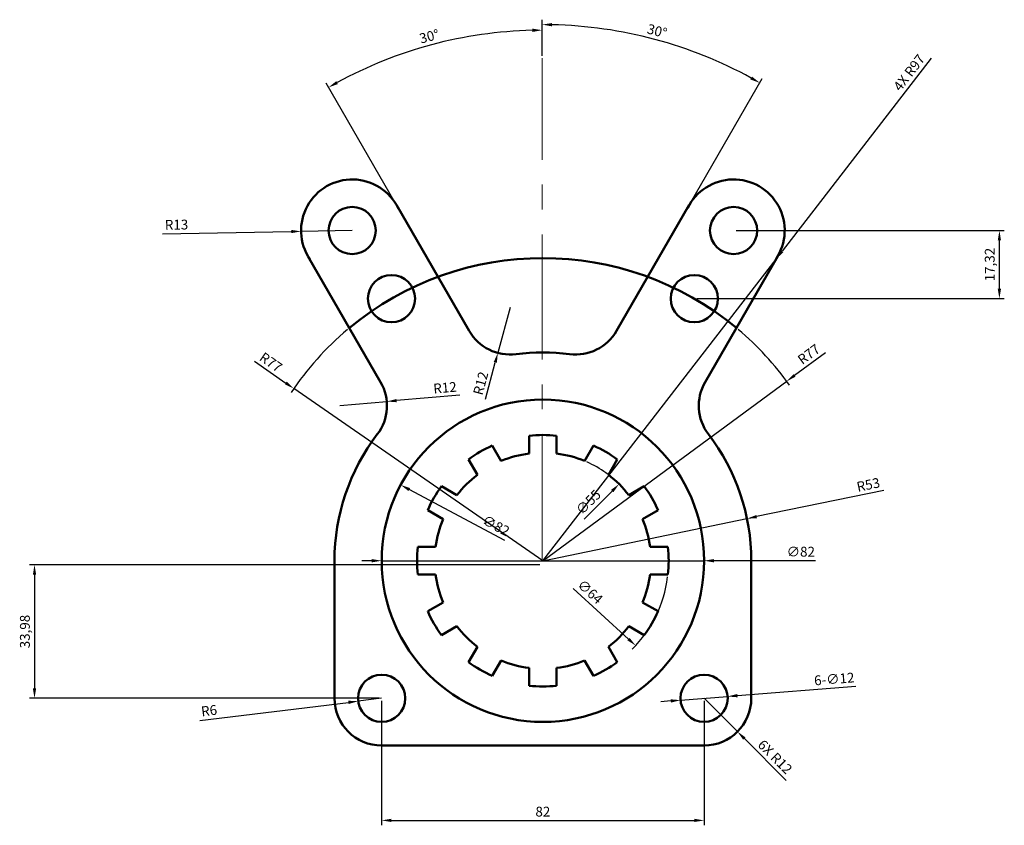
# Model space of a CAD drawing. Units: millimetres. Extents: x 2412 to 2662, y 1652 to 1857.
import ezdxf

# ---------------------------------------------------------------- set-up
doc = ezdxf.new("R2010")
doc.units = ezdxf.units.MM
doc.linetypes.add('CENTER', pattern=[50.8, 31.75, -6.35, 6.35, -6.35])
for name, color, linetype, lineweight in [('M-CNTR', 1, 'CENTER', 18), ('M-DIMS', 2, 'Continuous', 25), ('M-OUTL', 7, 'Continuous', 50)]:
    doc.layers.add(name, color=color, linetype=linetype, lineweight=lineweight)
doc.styles.get("Standard").update_dxf_attribs({"font": 'arial.ttf'})
doc.dimstyles.new('ISO-25', dxfattribs={"dimtxt": 2.5, "dimasz": 2.5, "dimexe": 1.25, "dimexo": 0.625, "dimtad": 1, "dimtxsty": 'Standard', "dimcen": 2.5, "dimadec": 0, "dimazin": 0, "dimtfac": 1, "dimtmove": 0, "dimatfit": 3, "dimfxl": 1, "dimarcsym": 0})

# ---------------------------------------------------------------- blocks, each defined once
blk = doc.blocks.new('*U1')
for p, q in [((-2.17, 3.5), (2.36, 3.5)), ((-2.17, -3.5), (2.36, -3.5))]:
    blk.add_line(p, q)
blk.add_arc((29.64, 0), 32, 173.7207, 186.2793)
blk = doc.blocks.new('*U2')
at = {"layer": 'M-OUTL', "color": 0, "linetype": 'ByBlock', "lineweight": -2, "transparency": 16777216}
for p, rotation in [((2545.03, 1748.83), 269.9999999999999), ((2530.22, 1744.86), 299.9999999999999), ((2559.85, 1744.86), 239.9999999999999), ((2519.37, 1734.01), 329.9999999999999), ((2570.7, 1734.01), 210), ((2574.67, 1719.2), 180), ((2519.37, 1704.38), 30), ((2570.7, 1704.38), 150), ((2530.22, 1693.53), 60), ((2559.85, 1693.53), 119.9999999999999), ((2545.03, 1689.56), 90.00000000000003)]:
    blk.add_blockref('*U1', p, dxfattribs=dict(at, rotation=rotation))
blk.add_blockref('*U1', (2515.4, 1719.2), dxfattribs=at)
blk = doc.blocks.new('*D3')
at = {"layer": 'Defpoints', "color": 0, "transparency": 16777216}
for p in [(2582.72, 1848.91), (2544.86, 1847.01), (2582.28, 1809.7), (2563.78, 1777.66), (2544.86, 1719.62)]:
    blk.add_point(p, dxfattribs=at)
at = {"layer": 'M-DIMS', "color": 0, "lineweight": -2, "transparency": 16777216}
for p, q in [((2544.86, 1847.64), (2544.86, 1856.84)), ((2582.59, 1810.24), (2600.83, 1841.84))]:
    blk.add_line(p, q, dxfattribs=at)
blk.add_arc((2544.86, 1744.89), 110.7, 61.2939, 88.7061, dxfattribs=at)
at = {"layer": 'M-DIMS', "color": 0, "transparency": 16777216}
for points in [[(2547.35, 1855.14), (2547.36, 1855.98), (2544.86, 1855.59)], [(2598.23, 1842.35), (2597.82, 1841.62), (2600.21, 1840.76)]]:
    blk.add_solid(points, dxfattribs=at)
at = {"layer": 'M-DIMS', "color": 0, "transparency": 16777216, "insert": (2574, 1853.66), "char_height": 2.5, "attachment_point": 5, "rotation": 345}
blk.add_mtext('30°', dxfattribs=at)
blk = doc.blocks.new('*D4')
at = {"layer": 'Defpoints', "color": 0, "transparency": 16777216}
for p in [(2525.99, 1852.52), (2544.86, 1847.01), (2507.79, 1809.7), (2526.29, 1777.66), (2544.86, 1719.62)]:
    blk.add_point(p, dxfattribs=at)
at = {"layer": 'M-DIMS', "color": 0, "lineweight": -2, "transparency": 16777216}
for p, q in [((2544.86, 1847.64), (2544.86, 1855.42)), ((2507.48, 1810.24), (2489.9, 1840.69))]:
    blk.add_line(p, q, dxfattribs=at)
blk.add_arc((2544.86, 1745.5), 108.66, 91.3182, 118.6818, dxfattribs=at)
at = {"layer": 'M-DIMS', "color": 0, "transparency": 16777216}
for points in [[(2542.35, 1854.56), (2542.36, 1853.72), (2544.86, 1854.17)], [(2492.91, 1840.47), (2492.5, 1841.2), (2490.52, 1839.61)]]:
    blk.add_solid(points, dxfattribs=at)
at = {"layer": 'M-DIMS', "color": 0, "transparency": 16777216, "insert": (2516.24, 1852.3), "char_height": 2.5, "attachment_point": 5, "rotation": 15}
blk.add_mtext('30°', dxfattribs=at)
blk = doc.blocks.new('*D5')
at = {"layer": 'Defpoints', "color": 0, "transparency": 16777216}
for p in [(2593.53, 1803.2), (2661.14, 1803.2), (2583.53, 1785.88)]:
    blk.add_point(p, dxfattribs=at)
at = {"layer": 'M-DIMS', "color": 0, "lineweight": -2, "transparency": 16777216}
for p, q in [((2594.16, 1803.2), (2662.39, 1803.2)), ((2661.14, 1788.38), (2661.14, 1800.7)), ((2584.16, 1785.88), (2662.39, 1785.88))]:
    blk.add_line(p, q, dxfattribs=at)
at = {"layer": 'M-DIMS', "color": 0, "transparency": 16777216}
for points in [[(2660.72, 1800.7), (2661.55, 1800.7), (2661.14, 1803.2)], [(2660.72, 1788.38), (2661.55, 1788.38), (2661.14, 1785.88)]]:
    blk.add_solid(points, dxfattribs=at)
at = {"layer": 'M-DIMS', "color": 0, "transparency": 16777216, "insert": (2659.01, 1794.54), "char_height": 2.5, "attachment_point": 5, "rotation": 90}
blk.add_mtext('17,32', dxfattribs=at)
blk = doc.blocks.new('*D6')
at = {"layer": 'Defpoints', "color": 0, "transparency": 16777216}
for p in [(2483.54, 1802.98), (2496.53, 1803.2)]:
    blk.add_point(p, dxfattribs=at)
at = {"layer": 'M-DIMS', "color": 0, "lineweight": -2, "transparency": 16777216}
for p, q in [((2496.53, 1803.2), (2483.54, 1802.98)), ((2448.29, 1802.4), (2481.04, 1802.94))]:
    blk.add_line(p, q, dxfattribs=at)
at = {"layer": 'M-DIMS', "color": 0, "transparency": 16777216}
blk.add_solid([(2481.03, 1803.36), (2481.04, 1802.53), (2483.54, 1802.98)], dxfattribs=at)
at = {"layer": 'M-DIMS', "color": 0, "transparency": 16777216, "insert": (2451.87, 1804.36), "char_height": 2.5, "attachment_point": 5, "rotation": 0.9546}
blk.add_mtext('R13', dxfattribs=at)
blk = doc.blocks.new('*D7')
at = {"layer": 'Defpoints', "color": 0, "transparency": 16777216}
for p in [(2493.38, 1758.66), (2505.34, 1759.71)]:
    blk.add_point(p, dxfattribs=at)
at = {"layer": 'M-DIMS', "color": 0, "lineweight": -2, "transparency": 16777216}
for p, q in [((2523.91, 1761.34), (2507.83, 1759.93)), ((2493.38, 1758.66), (2505.34, 1759.71))]:
    blk.add_line(p, q, dxfattribs=at)
at = {"layer": 'M-DIMS', "color": 0, "transparency": 16777216}
blk.add_solid([(2507.79, 1760.34), (2507.87, 1759.51), (2505.34, 1759.71)], dxfattribs=at)
at = {"layer": 'M-DIMS', "color": 0, "transparency": 16777216, "insert": (2520.16, 1762.89), "char_height": 2.5, "attachment_point": 5, "rotation": 5.0173}
blk.add_mtext('R12', dxfattribs=at)
blk = doc.blocks.new('*D8')
at = {"layer": 'Defpoints', "color": 0, "transparency": 16777216}
for p in [(2544.86, 1718.17), (2415.74, 1684.2), (2504.03, 1684.2)]:
    blk.add_point(p, dxfattribs=at)
at = {"layer": 'M-DIMS', "color": 0, "lineweight": -2, "transparency": 16777216}
for p, q in [((2544.23, 1718.17), (2414.49, 1718.17)), ((2415.74, 1715.67), (2415.74, 1686.7)), ((2503.41, 1684.2), (2414.49, 1684.2))]:
    blk.add_line(p, q, dxfattribs=at)
at = {"layer": 'M-DIMS', "color": 0, "transparency": 16777216}
for points in [[(2415.33, 1715.67), (2416.16, 1715.67), (2415.74, 1718.17)], [(2415.33, 1686.7), (2416.16, 1686.7), (2415.74, 1684.2)]]:
    blk.add_solid(points, dxfattribs=at)
at = {"layer": 'M-DIMS', "color": 0, "transparency": 16777216, "insert": (2413.62, 1701.18), "char_height": 2.5, "attachment_point": 5, "rotation": 90}
blk.add_mtext('33,98', dxfattribs=at)
blk = doc.blocks.new('*D9')
at = {"layer": 'Defpoints', "color": 0, "transparency": 16777216}
for p in [(2498.08, 1683.47), (2504.03, 1684.2)]:
    blk.add_point(p, dxfattribs=at)
at = {"layer": 'M-DIMS', "color": 0, "lineweight": -2, "transparency": 16777216}
for p, q in [((2457.79, 1678.54), (2495.6, 1683.16)), ((2504.03, 1684.2), (2498.08, 1683.47))]:
    blk.add_line(p, q, dxfattribs=at)
at = {"layer": 'M-DIMS', "color": 0, "transparency": 16777216}
blk.add_solid([(2495.55, 1683.58), (2495.65, 1682.75), (2498.08, 1683.47)], dxfattribs=at)
at = {"layer": 'M-DIMS', "color": 0, "transparency": 16777216, "insert": (2460.18, 1680.75), "char_height": 2.5, "attachment_point": 5, "rotation": 6.9713}
blk.add_mtext('R6', dxfattribs=at)
blk = doc.blocks.new('*D10')
at = {"layer": 'Defpoints', "color": 0, "transparency": 16777216}
for p in [(2504.03, 1684.2), (2586.03, 1684.2), (2586.03, 1653.13)]:
    blk.add_point(p, dxfattribs=at)
at = {"layer": 'M-DIMS', "color": 0, "lineweight": -2, "transparency": 16777216}
for p, q in [((2504.03, 1683.57), (2504.03, 1651.88)), ((2586.03, 1683.57), (2586.03, 1651.88)), ((2506.53, 1653.13), (2583.53, 1653.13))]:
    blk.add_line(p, q, dxfattribs=at)
at = {"layer": 'M-DIMS', "color": 0, "transparency": 16777216}
for points in [[(2506.53, 1653.55), (2506.53, 1652.72), (2504.03, 1653.13)], [(2583.53, 1653.55), (2583.53, 1652.72), (2586.03, 1653.13)]]:
    blk.add_solid(points, dxfattribs=at)
at = {"layer": 'M-DIMS', "color": 0, "transparency": 16777216, "insert": (2545.03, 1655.04), "char_height": 2.5, "attachment_point": 5}
blk.add_mtext('82', dxfattribs=at)
blk = doc.blocks.new('*D11')
at = {"layer": 'Defpoints', "color": 0, "transparency": 16777216}
for p in [(2580.05, 1683.72), (2592.02, 1684.67)]:
    blk.add_point(p, dxfattribs=at)
at = {"layer": 'M-DIMS', "color": 0, "lineweight": -2, "transparency": 16777216}
for p, q in [((2624.61, 1687.24), (2594.51, 1684.86)), ((2577.56, 1683.53), (2575.07, 1683.33)), ((2580.05, 1683.72), (2592.02, 1684.67))]:
    blk.add_line(p, q, dxfattribs=at)
at = {"layer": 'M-DIMS', "color": 0, "transparency": 16777216}
for points in [[(2594.48, 1685.28), (2594.54, 1684.45), (2592.02, 1684.67)], [(2577.53, 1683.94), (2577.59, 1683.11), (2580.05, 1683.72)]]:
    blk.add_solid(points, dxfattribs=at)
at = {"layer": 'M-DIMS', "color": 0, "transparency": 16777216, "insert": (2619.16, 1688.79), "char_height": 2.5, "attachment_point": 5, "rotation": 4.5152}
blk.add_mtext('6-∅12', dxfattribs=at)
blk = doc.blocks.new('*D12')
at = {"layer": 'Defpoints', "color": 0, "transparency": 16777216}
for p in [(2536.69, 1783.66), (2533.58, 1772.07)]:
    blk.add_point(p, dxfattribs=at)
at = {"layer": 'M-DIMS', "color": 0, "lineweight": -2, "transparency": 16777216}
for p, q in [((2536.69, 1783.66), (2533.58, 1772.07)), ((2530.41, 1760.29), (2532.93, 1769.65))]:
    blk.add_line(p, q, dxfattribs=at)
at = {"layer": 'M-DIMS', "color": 0, "transparency": 16777216}
blk.add_solid([(2532.53, 1769.76), (2533.33, 1769.54), (2533.58, 1772.07)], dxfattribs=at)
at = {"layer": 'M-DIMS', "color": 0, "transparency": 16777216, "insert": (2529.53, 1764.25), "char_height": 2.5, "attachment_point": 5, "rotation": 74.9785}
blk.add_mtext('R12', dxfattribs=at)
blk = doc.blocks.new('*D13')
at = {"layer": 'Defpoints', "color": 0, "transparency": 16777216}
for p in [(2596.94, 1729.9), (2545.03, 1719.2)]:
    blk.add_point(p, dxfattribs=at)
at = {"layer": 'M-DIMS', "color": 0, "lineweight": -2, "transparency": 16777216}
for p, q in [((2631.78, 1737.09), (2599.39, 1730.41)), ((2545.03, 1719.2), (2596.94, 1729.9))]:
    blk.add_line(p, q, dxfattribs=at)
at = {"layer": 'M-DIMS', "color": 0, "transparency": 16777216}
blk.add_solid([(2599.31, 1730.82), (2599.47, 1730), (2596.94, 1729.9)], dxfattribs=at)
at = {"layer": 'M-DIMS', "color": 0, "transparency": 16777216, "insert": (2627.86, 1738.22), "char_height": 2.5, "attachment_point": 5, "rotation": 11.6561}
blk.add_mtext('R53', dxfattribs=at)
blk = doc.blocks.new('*D14')
at = {"layer": 'Defpoints', "color": 0, "transparency": 16777216}
for p in [(2521.43, 1740.8), (2568.64, 1697.59)]:
    blk.add_point(p, dxfattribs=at)
at = {"layer": 'M-DIMS', "color": 0, "lineweight": -2, "transparency": 16777216}
blk.add_line((2552.73, 1712.16), (2566.8, 1699.28), dxfattribs=at)
blk.add_arc((2545.03, 1719.2), 32, 315.2921, 352.6017, dxfattribs=at)
at = {"layer": 'M-DIMS', "color": 0, "transparency": 16777216}
blk.add_solid([(2567.08, 1699.58), (2566.51, 1698.97), (2568.64, 1697.59)], dxfattribs=at)
at = {"layer": 'M-DIMS', "color": 0, "transparency": 16777216, "insert": (2556.84, 1711.06), "char_height": 2.5, "attachment_point": 5, "rotation": 317.5302}
blk.add_mtext('∅64', dxfattribs=at)
blk = doc.blocks.new('*D15')
at = {"layer": 'Defpoints', "color": 0, "transparency": 16777216}
for p in [(2508.85, 1738.48), (2581.22, 1699.91)]:
    blk.add_point(p, dxfattribs=at)
at = {"layer": 'M-DIMS', "color": 0, "lineweight": -2, "transparency": 16777216}
blk.add_line((2535.36, 1724.35), (2511.06, 1737.3), dxfattribs=at)
at = {"layer": 'M-DIMS', "color": 0, "transparency": 16777216}
blk.add_solid([(2511.25, 1737.67), (2510.86, 1736.93), (2508.85, 1738.48)], dxfattribs=at)
at = {"layer": 'M-DIMS', "color": 0, "transparency": 16777216, "insert": (2532.96, 1727.86), "char_height": 2.5, "attachment_point": 5, "rotation": 331.9485}
blk.add_mtext('∅82', dxfattribs=at)
blk = doc.blocks.new('*D16')
at = {"layer": 'Defpoints', "color": 0, "transparency": 16777216}
for p in [(2564.42, 1738.7), (2525.65, 1699.69)]:
    blk.add_point(p, dxfattribs=at)
at = {"layer": 'M-DIMS', "color": 0, "lineweight": -2, "transparency": 16777216}
blk.add_line((2555.56, 1729.78), (2562.66, 1736.92), dxfattribs=at)
blk.add_arc((2545.03, 1719.2), 27.5, 42.562, 66.0098, dxfattribs=at)
at = {"layer": 'M-DIMS', "color": 0, "transparency": 16777216}
blk.add_solid([(2562.37, 1737.22), (2562.96, 1736.63), (2564.42, 1738.7)], dxfattribs=at)
at = {"layer": 'M-DIMS', "color": 0, "transparency": 16777216, "insert": (2556.83, 1733.86), "char_height": 2.5, "attachment_point": 5, "rotation": 45.1664}
blk.add_mtext('∅55', dxfattribs=at)
blk = doc.blocks.new('*D17')
at = {"layer": 'Defpoints', "color": 0, "transparency": 16777216}
for p in [(2481.7, 1762.99), (2545.03, 1719.2)]:
    blk.add_point(p, dxfattribs=at)
at = {"layer": 'M-DIMS', "color": 0, "lineweight": -2, "transparency": 16777216}
for p, q in [((2471.65, 1769.95), (2479.65, 1764.41)), ((2545.03, 1719.2), (2481.7, 1762.99))]:
    blk.add_line(p, q, dxfattribs=at)
blk.add_arc((2545.03, 1719.2), 77, 130.1849, 146.2641, dxfattribs=at)
at = {"layer": 'M-DIMS', "color": 0, "transparency": 16777216}
blk.add_solid([(2479.88, 1764.76), (2479.41, 1764.07), (2481.7, 1762.99)], dxfattribs=at)
at = {"layer": 'M-DIMS', "color": 0, "transparency": 16777216, "insert": (2475.69, 1769.43), "char_height": 2.5, "attachment_point": 5, "rotation": 325.334}
blk.add_mtext('R77', dxfattribs=at)
blk = doc.blocks.new('*D18')
at = {"layer": 'Defpoints', "color": 0, "transparency": 16777216}
for p in [(2607.04, 1764.85), (2545.03, 1719.2)]:
    blk.add_point(p, dxfattribs=at)
at = {"layer": 'M-DIMS', "color": 0, "lineweight": -2, "transparency": 16777216}
for p, q in [((2616.88, 1772.1), (2609.05, 1766.33)), ((2545.03, 1719.2), (2607.04, 1764.85))]:
    blk.add_line(p, q, dxfattribs=at)
blk.add_arc((2545.03, 1719.2), 77, 35.4331, 49.8151, dxfattribs=at)
at = {"layer": 'M-DIMS', "color": 0, "transparency": 16777216}
blk.add_solid([(2608.81, 1766.67), (2609.3, 1766), (2607.04, 1764.85)], dxfattribs=at)
at = {"layer": 'M-DIMS', "color": 0, "transparency": 16777216, "insert": (2612.86, 1771.47), "char_height": 2.5, "attachment_point": 5, "rotation": 36.3632}
blk.add_mtext('R77', dxfattribs=at)
blk = doc.blocks.new('*D19')
at = {"layer": 'Defpoints', "color": 0, "transparency": 16777216}
for p in [(2504.03, 1719.2), (2586.03, 1719.2)]:
    blk.add_point(p, dxfattribs=at)
at = {"layer": 'M-DIMS', "color": 0, "lineweight": -2, "transparency": 16777216}
for p, q in [((2501.53, 1719.2), (2499.03, 1719.2)), ((2504.03, 1719.2), (2586.03, 1719.2)), ((2614.4, 1719.2), (2588.53, 1719.2))]:
    blk.add_line(p, q, dxfattribs=at)
at = {"layer": 'M-DIMS', "color": 0, "transparency": 16777216}
for points in [[(2501.53, 1719.61), (2501.53, 1718.78), (2504.03, 1719.2)], [(2588.53, 1719.61), (2588.53, 1718.78), (2586.03, 1719.2)]]:
    blk.add_solid(points, dxfattribs=at)
at = {"layer": 'M-DIMS', "color": 0, "transparency": 16777216, "insert": (2610.63, 1721.17), "char_height": 2.5, "attachment_point": 5, "rotation": 0.0005}
blk.add_mtext('∅82', dxfattribs=at)
blk = doc.blocks.new('*D20')
at = {"layer": 'Defpoints', "color": 0, "transparency": 16777216}
for p in [(2586.03, 1684.2), (2594.52, 1675.71)]:
    blk.add_point(p, dxfattribs=at)
at = {"layer": 'M-DIMS', "color": 0, "lineweight": -2, "transparency": 16777216}
for p, q in [((2586.03, 1684.2), (2594.52, 1675.71)), ((2606.95, 1663.28), (2596.29, 1673.94))]:
    blk.add_line(p, q, dxfattribs=at)
at = {"layer": 'M-DIMS', "color": 0, "transparency": 16777216}
blk.add_solid([(2596.58, 1674.24), (2595.99, 1673.65), (2594.52, 1675.71)], dxfattribs=at)
at = {"layer": 'M-DIMS', "color": 0, "transparency": 16777216, "insert": (2603.85, 1669.07), "char_height": 2.5, "attachment_point": 5, "rotation": 314.998}
blk.add_mtext('6X R12', dxfattribs=at)
blk = doc.blocks.new('*D21')
at = {"layer": 'Defpoints', "color": 0, "transparency": 16777216}
for p in [(2604.34, 1795.95), (2545.03, 1719.2)]:
    blk.add_point(p, dxfattribs=at)
at = {"layer": 'M-DIMS', "color": 0, "lineweight": -2, "transparency": 16777216}
for p, q in [((2643.81, 1847.03), (2605.87, 1797.93)), ((2545.03, 1719.2), (2604.34, 1795.95))]:
    blk.add_line(p, q, dxfattribs=at)
at = {"layer": 'M-DIMS', "color": 0, "transparency": 16777216}
blk.add_solid([(2605.54, 1798.18), (2606.2, 1797.67), (2604.34, 1795.95)], dxfattribs=at)
at = {"layer": 'M-DIMS', "color": 0, "transparency": 16777216, "insert": (2638.43, 1843.17), "char_height": 2.5, "attachment_point": 5, "rotation": 52.3067}
blk.add_mtext('4X R97', dxfattribs=at)

msp = doc.modelspace()

# ---------------------------------------------------------------- linework, layer by layer
at = {"layer": 'M-CNTR'}
for p, q in [((2544.857, 1719.619), (2544.857, 1847.014)), ((2545.035, 1719.196), (2545.035, 1719.196))]:
    msp.add_line(p, q, dxfattribs=at)
at = {"layer": 'M-OUTL'}
for p, q in [((2526.293, 1777.657), (2507.793, 1809.7)), ((2563.777, 1777.657), (2582.277, 1809.7)), ((2503.777, 1764.657), (2485.277, 1796.7)), ((2586.293, 1764.657), (2604.793, 1796.7)), ((2492.035, 1684.196), (2492.035, 1719.196)), ((2598.035, 1684.196), (2598.035, 1719.196)), ((2504.035, 1672.196), (2586.035, 1672.196))]:
    msp.add_line(p, q, dxfattribs=at)
for centre, radius in [((2496.535, 1803.2), 6), ((2593.535, 1803.2), 6), ((2506.535, 1785.88), 6), ((2583.535, 1785.88), 6), ((2545.035, 1719.196), 41), ((2504.035, 1684.196), 6), ((2586.035, 1684.196), 6)]:
    msp.add_circle(centre, radius, dxfattribs=at)
for centre, radius, start, end in [((2496.535, 1803.2), 13, 26.15771, 213.84229), ((2593.535, 1803.2), 13, 326.15771, 153.84229), ((2545.035, 1719.196), 97, 112.29801, 112.31543), ((2545.035, 1719.196), 97, 67.68457, 67.70199), ((2545.035, 1719.196), 97, 127.68457, 127.70199), ((2545.035, 1719.196), 77, 50.28013, 129.71987), ((2545.035, 1719.196), 97, 52.29801, 52.31543), ((2536.686, 1783.657), 12, 210, 277.38014), ((2553.384, 1783.657), 12, 262.61986, 330), ((2545.035, 1719.196), 53, 82.61986, 97.38014), ((2493.384, 1758.657), 12, 322.61986, 30), ((2596.686, 1758.657), 12, 150, 217.38014), ((2545.035, 1719.196), 53, 142.61986, 180), ((2545.035, 1719.196), 53, 0, 37.38014), ((2545.035, 1719.196), 27.5, 97.31202, 112.68798), ((2545.035, 1719.196), 27.5, 67.31202, 82.68798), ((2545.035, 1719.196), 27.5, 127.31202, 142.68798), ((2545.035, 1719.196), 27.5, 37.31202, 52.68798), ((2545.035, 1719.196), 27.5, 157.31202, 172.68798), ((2545.035, 1719.196), 27.5, 7.31202, 22.68798), ((2545.035, 1719.196), 27.5, 187.31202, 202.68798), ((2545.035, 1719.196), 27.5, 337.31202, 352.68798), ((2545.035, 1719.196), 27.5, 217.31202, 232.68798), ((2545.035, 1719.196), 27.5, 307.31202, 322.68798), ((2545.035, 1719.196), 27.5, 247.31202, 262.68798), ((2545.035, 1719.196), 27.5, 277.31202, 292.68798), ((2504.035, 1684.196), 12, 180, 270), ((2586.035, 1684.196), 12, 270, 0)]:
    msp.add_arc(centre, radius, start, end, dxfattribs=at)

# ---------------------------------------------------------------- block references
msp.add_blockref('*U2', (0, 0), dxfattribs=at)

# ---------------------------------------------------------------- dimensions: what is measured, and where the dimension line sits
at = {"layer": 'M-DIMS'}
for base, line1, picture, middle in [((2582.719, 1848.914), ((2563.777, 1777.657), (2582.277, 1809.7)), '*D3', (2574.001, 1853.655)), ((2525.987, 1852.517), ((2526.293, 1777.657), (2507.793, 1809.7)), '*D4', (2516.24, 1852.303))]:
    dim = msp.add_angular_dim_2l(base=base, line1=line1, line2=((2544.857, 1719.619), (2544.857, 1847.014)), dimstyle='ISO-25', override={"dimclrd": 0, "dimclre": 0, "dimclrt": 0}, dxfattribs=at)
    dim.commit()
    dim.dimension.update_dxf_attribs({"geometry": picture, "text_midpoint": middle})
dim = msp.add_radius_dim(center=(2545.035, 1719.196), mpoint=(2604.344, 1795.951), text='4X <>', dimstyle='ISO-25', override={"dimdec": 0, "dimlfac": 1, "dimrnd": 0, "dimzin": 0, "dimdsep": 46, "dimlunit": 2}, dxfattribs=at)
dim.commit()
dim.dimension.update_dxf_attribs({"geometry": '*D21', "text_midpoint": (2639.93, 1842.005), "dimtype": 164})
for center, mpoint, picture, middle in [((2496.535, 1803.2), (2483.537, 1802.984), '*D6', (2451.902, 1802.456)), ((2493.384, 1758.657), (2505.338, 1759.707), '*D7', (2520.321, 1761.022)), ((2545.035, 1719.196), (2596.942, 1729.904), '*D13', (2628.243, 1736.361)), ((2504.035, 1684.196), (2498.079, 1683.467), '*D9', (2460.41, 1678.861))]:
    dim = msp.add_radius_dim(center=center, mpoint=mpoint, dimstyle='ISO-25', override={"dimclrd": 0, "dimclre": 0, "dimclrt": 0}, dxfattribs=at)
    dim.commit()
    dim.dimension.update_dxf_attribs({"geometry": picture, "text_midpoint": middle, "dimtype": 164})
for base, p1, p2, picture, middle in [((2661.136, 1803.2), (2583.535, 1785.88), (2593.535, 1803.2), '*D5', (2659.009, 1794.54)), ((2415.7425, 1684.1956), (2544.8567, 1718.171), (2504.035, 1684.1956), '*D8', (2413.6151, 1701.1833))]:
    dim = msp.add_linear_dim(base=base, p1=p1, p2=p2, angle=90, dimstyle='ISO-25', override={"dimclrd": 0, "dimclre": 0, "dimclrt": 0}, dxfattribs=at)
    dim.commit()
    dim.dimension.update_dxf_attribs({"geometry": picture, "text_midpoint": middle})
for center, mpoint, picture, middle in [((2536.686, 1783.657), (2533.575, 1772.067), '*D12', (2529.531, 1764.249)), ((2545.035, 1719.196), (2481.704, 1762.993), '*D17', (2475.687, 1769.433)), ((2545.035, 1719.196), (2607.041, 1764.849), '*D18', (2612.864, 1771.465))]:
    dim = msp.add_radius_dim(center=center, mpoint=mpoint, dimstyle='ISO-25', override={"dimclrd": 0, "dimclre": 0, "dimclrt": 0}, dxfattribs=at)
    dim.commit()
    dim.dimension.update_dxf_attribs({"geometry": picture, "text_midpoint": middle})
for p1, p2, override, picture, middle in [((2525.646, 1699.694), (2564.424, 1738.697), {"dimclrd": 0, "dimclre": 0, "dimclrt": 0}, '*D16', (2558.23, 1732.468)), ((2521.431, 1740.802), (2568.639, 1697.589), {"dimclrd": 0, "dimclre": 0, "dimclrt": 0}, '*D14', (2555.507, 1709.61)), ((2581.219, 1699.915), (2508.851, 1738.476), {"dimclrd": 0, "dimclre": 0, "dimclrt": 0}, '*D15', (2532.035, 1726.123)), ((2504.035, 1719.195), (2586.035, 1719.196), {"dimdec": 0, "dimlfac": 1, "dimrnd": 0, "dimzin": 0, "dimdsep": 46, "dimlunit": 2}, '*D19', (2610.635, 1719.196))]:
    dim = msp.add_diameter_dim_2p(p1=p1, p2=p2, dimstyle='ISO-25', override=override, dxfattribs=at)
    dim.commit()
    dim.dimension.update_dxf_attribs({"geometry": picture, "text_midpoint": middle, "dimtype": 163})
dim = msp.add_diameter_dim_2p(p1=(2580.054, 1683.723), p2=(2592.016, 1684.668), text='6-<>', dimstyle='ISO-25', override={"dimclrd": 0, "dimclre": 0, "dimclrt": 0}, dxfattribs=at)
dim.commit()
dim.dimension.update_dxf_attribs({"geometry": '*D11', "text_midpoint": (2619.311, 1686.823), "dimtype": 163})
dim = msp.add_linear_dim(base=(2586.035, 1653.134), p1=(2504.035, 1684.196), p2=(2586.035, 1684.196), dimstyle='ISO-25', override={"dimclrd": 0, "dimclre": 0, "dimclrt": 0}, dxfattribs=at)
dim.commit()
dim.dimension.update_dxf_attribs({"geometry": '*D10', "text_midpoint": (2545.035, 1655.036)})
dim = msp.add_radius_dim(center=(2586.035, 1684.196), mpoint=(2594.52, 1675.71), text='6X <>', dimstyle='ISO-25', override={"dimdec": 0, "dimlfac": 1, "dimrnd": 0, "dimzin": 0, "dimdsep": 46, "dimlunit": 2}, dxfattribs=at)
dim.commit()
dim.dimension.update_dxf_attribs({"geometry": '*D20', "text_midpoint": (2603.849, 1669.07)})

doc.saveas('drawing.dxf')
